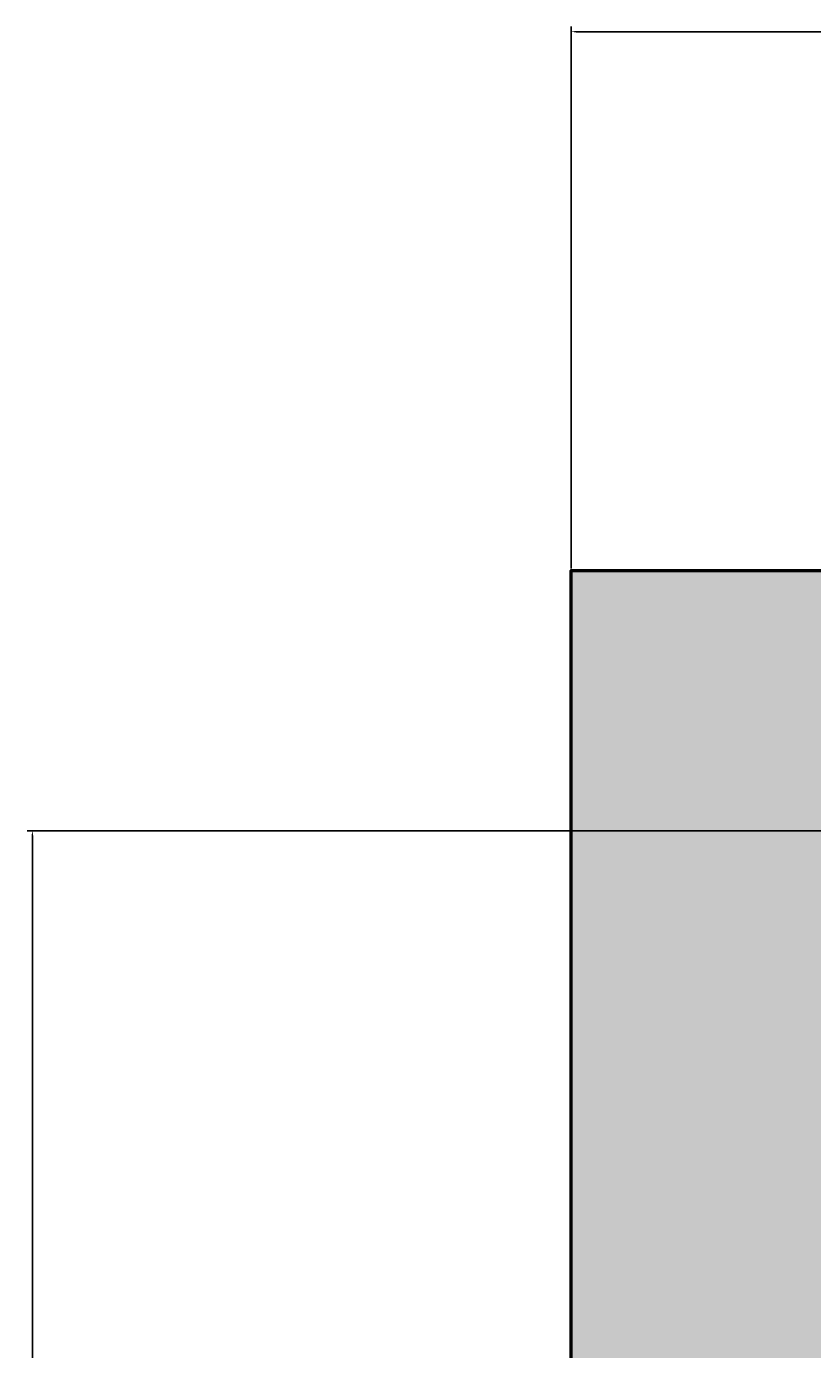
# Model space of a CAD drawing. Units: inches. Extents: x 2231 to 2461, y 2045 to 2455.
# Tile 74 of 95: x 2231 to 2258, y 2409 to 2455. Entities that reach past the tile are written whole.
import ezdxf

# ---------------------------------------------------------------- set-up
doc = ezdxf.new("R2010")
doc.units = ezdxf.units.IN
doc.layers.add('A-ANNO-DIMS', color=2, linetype='Continuous', lineweight=18)
doc.layers.add('A-WALL', color=7, linetype='Continuous', lineweight=50)
doc.layers.add('A-WALL-PATT', color=18, linetype='Continuous', lineweight=13, true_color=0x000000)
doc.styles.get("Standard").update_dxf_attribs({"font": 'arial.ttf'})
doc.dimstyles.get("Standard").update_dxf_attribs({"dimtxt": 0.18, "dimasz": 0.18, "dimexe": 0.18, "dimexo": 0.0625, "dimgap": 0.09, "dimtad": 0, "dimtih": 1, "dimtoh": 1, "dimdec": 4, "dimzin": 0, "dimdsep": 46, "dimtxsty": 'Standard', "dimcen": 0.09, "dimadec": 0, "dimazin": 0, "dimtfac": 1, "dimtdec": 4, "dimtofl": 0, "dimtmove": 0, "dimatfit": 3, "dimfxl": 1, "dimtolj": 1, "dimtzin": 0, "dimarcsym": 0})

# ---------------------------------------------------------------- blocks, each defined once
blk = doc.blocks.new('*D37')
at = {"layer": 'A-ANNO-DIMS', "color": 0, "lineweight": -2, "transparency": 16777216}
for p, q in [((2258.731, 2426.833), (2230.981, 2426.833)), ((2231.161, 2426.653), (2231.161, 2367.015)), ((2231.161, 2307.013), (2231.161, 2366.651)), ((2258.731, 2306.833), (2230.981, 2306.833))]:
    blk.add_line(p, q, dxfattribs=at)
at = {"layer": 'A-ANNO-DIMS', "color": 0, "transparency": 16777216}
for points in [[(2231.131, 2426.653), (2231.191, 2426.653), (2231.161, 2426.833)], [(2231.131, 2307.013), (2231.191, 2307.013), (2231.161, 2306.833)]]:
    blk.add_solid(points, dxfattribs=at)
at = {"layer": 'Defpoints', "color": 0, "transparency": 16777216}
for p in [(2231.161, 2426.833), (2258.794, 2426.833), (2258.794, 2306.833)]:
    blk.add_point(p, dxfattribs=at)
at = {"layer": 'A-ANNO-DIMS', "color": 0, "transparency": 16777216, "insert": (2231.161, 2366.833), "char_height": 0.18, "attachment_point": 5}
blk.add_mtext('\\A1;120', dxfattribs=at)
blk = doc.blocks.new('*D55')
at = {"layer": 'A-ANNO-DIMS', "color": 0, "lineweight": -2, "transparency": 16777216}
for p, q in [((2249.794, 2435.895), (2249.794, 2454.645)), ((2249.974, 2454.465), (2267.413, 2454.465)), ((2285.64, 2454.465), (2268.2, 2454.465)), ((2285.82, 2435.895), (2285.82, 2454.645))]:
    blk.add_line(p, q, dxfattribs=at)
at = {"layer": 'A-ANNO-DIMS', "color": 0, "transparency": 16777216}
for points in [[(2249.974, 2454.495), (2249.974, 2454.435), (2249.794, 2454.465)], [(2285.64, 2454.495), (2285.64, 2454.435), (2285.82, 2454.465)]]:
    blk.add_solid(points, dxfattribs=at)
at = {"layer": 'Defpoints', "color": 0, "transparency": 16777216}
for p in [(2285.82, 2454.465), (2249.794, 2435.833), (2285.82, 2435.833)]:
    blk.add_point(p, dxfattribs=at)
at = {"layer": 'A-ANNO-DIMS', "color": 0, "transparency": 16777216, "insert": (2267.807, 2454.465), "char_height": 0.18, "attachment_point": 5}
blk.add_mtext('\\A1;36.03', dxfattribs=at)

msp = doc.modelspace()

# ---------------------------------------------------------------- hatches: boundary and pattern name
at = {"layer": 'A-WALL-PATT'}
h = msp.add_hatch(color=256, dxfattribs=at)
h.dxf.hatch_style = 1
h.paths.add_polyline_path([(2441.7935, 2269.1535), (2432.7935, 2269.1535), (2432.7935, 2186.8328), (2396.7935, 2186.8328), (2396.7935, 2286.8328), (2394.7935, 2286.8328), (2394.7935, 2186.8328), (2334.7935, 2186.8328), (2334.7935, 2182.8328), (2432.7935, 2182.8328), (2432.7935, 2072.8328), (2416.6639, 2072.8328), (2416.6639, 2063.8328), (2441.7935, 2063.8328)])
h.paths.add_polyline_path([(2368.6639, 2072.8328), (2367.04, 2072.8328), (2330.7942, 2072.8328), (2330.7397, 2063.8328), (2368.6639, 2063.8328)])
h.paths.add_polyline_path([(2300.7392, 2068.3328), (2300.7392, 2072.8328), (2298.7935, 2072.8328), (2294.7935, 2072.8328), (2258.7935, 2072.8328), (2258.7935, 2120.8328), (2294.7935, 2120.8328), (2298.7935, 2120.8328), (2298.7935, 2128.8328), (2294.7935, 2128.8328), (2294.7935, 2124.8328), (2258.7935, 2124.8328), (2258.7935, 2182.8328), (2294.7935, 2182.8328), (2294.7935, 2174.8328), (2298.7935, 2174.8328), (2298.7935, 2182.8328), (2304.7935, 2182.8328), (2304.7935, 2186.8328), (2258.7935, 2186.8328), (2258.7935, 2221.999), (2249.7935, 2221.999), (2249.7935, 2063.8328), (2300.7392, 2063.8328)])
h.paths.add_polyline_path([(2391.9338, 2435.8328), (2333.82, 2435.8328), (2333.82, 2426.8328), (2368.7935, 2426.8328), (2368.7935, 2374.9508), (2368.7935, 2370.8328), (2372.3935, 2370.8328), (2372.7935, 2370.8328), (2372.7935, 2426.8328), (2391.9338, 2426.8328)])
h.paths.add_polyline_path([(2441.7935, 2435.8328), (2415.9338, 2435.8328), (2415.9338, 2426.8328), (2432.7935, 2426.8328), (2432.7935, 2334.8328), (2372.7935, 2334.8328), (2372.7935, 2346.8328), (2368.7935, 2346.8328), (2368.7935, 2306.8328), (2360.7935, 2306.8328), (2360.7935, 2302.8328), (2368.7935, 2302.8328), (2372.7935, 2302.8328), (2372.7935, 2330.8328), (2432.7935, 2330.8328), (2432.7935, 2317.1535), (2441.7935, 2317.1535)])
h.paths.add_polyline_path([(2285.82, 2435.8328), (2249.7935, 2435.8328), (2249.7935, 2269.999), (2258.7935, 2269.999), (2258.7935, 2302.8328), (2318.8168, 2302.8328), (2330.7935, 2302.8328), (2330.7935, 2306.8328), (2258.7935, 2306.8328), (2258.7935, 2426.8328), (2285.82, 2426.8328)])

# ---------------------------------------------------------------- linework, layer by layer
at = {"layer": 'A-WALL'}
msp.add_lwpolyline([(2300.7392, 2063.8328), (2249.7935, 2063.8328), (2249.7935, 2435.8328), (2441.7935, 2435.8328), (2441.7935, 2063.8328), (2330.7397, 2063.8328)], dxfattribs=at)

# ---------------------------------------------------------------- dimensions: what is measured, and where the dimension line sits
at = {"layer": 'A-ANNO-DIMS'}
dim = msp.add_linear_dim(base=(2285.82, 2454.4653), p1=(2249.7935, 2435.8328), p2=(2285.82, 2435.8328), dimstyle='Standard', override={"dimdec": 2, "dimlfac": 1, "dimrnd": 0, "dimzin": 0, "dimdsep": 46, "dimlunit": 2}, dxfattribs=at)
dim.commit()
dim.dimension.update_dxf_attribs({"geometry": '*D55', "text_midpoint": (2267.8067, 2454.4653)})
dim = msp.add_linear_dim(base=(2231.161, 2426.8328), p1=(2258.7935, 2306.8328), p2=(2258.7935, 2426.8328), angle=90, dimstyle='Standard', override={"dimdec": 0, "dimlfac": 1, "dimrnd": 0, "dimzin": 0, "dimdsep": 46, "dimlunit": 2}, dxfattribs=at)
dim.commit()
dim.dimension.update_dxf_attribs({"geometry": '*D37', "text_midpoint": (2231.161, 2366.8328)})

doc.saveas('drawing.dxf')
